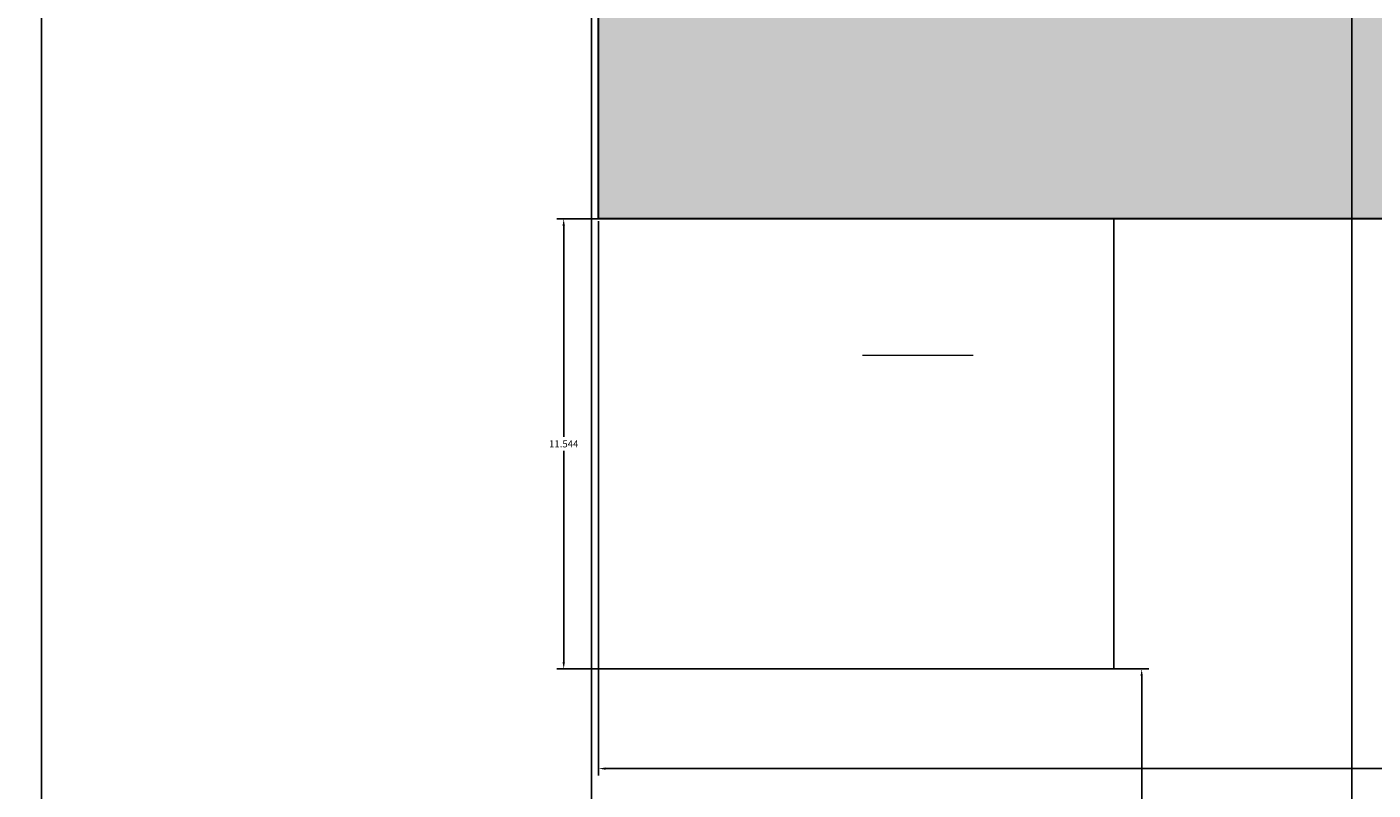
# Model space of a CAD drawing. Units: millimetres. Extents: x -8 to 285, y 5 to 221.
# Tile 11 of 30: x -8 to 27, y 131 to 150. Entities that reach past the tile are written whole.
import ezdxf

# ---------------------------------------------------------------- set-up
doc = ezdxf.new("R2010")
doc.units = ezdxf.units.MM
for name, color, linetype, lineweight in [('A-ANNO-DIMS', 2, 'Continuous', 18), ('E-ANNO-SYMB', 7, 'Continuous', 18), ('E-EQPM-PATT', 252, 'Continuous', 13), ('E-POWR-DC-NEG', 3, 'Continuous', 25), ('E-POWR-PV', 7, 'Continuous', 30)]:
    doc.layers.add(name, color=color, linetype=linetype, lineweight=lineweight)
doc.styles.get("Standard").update_dxf_attribs({"font": 'arial.ttf'})
doc.dimstyles.get("Standard").update_dxf_attribs({"dimtxt": 0.18, "dimasz": 0.18, "dimexe": 0.18, "dimexo": 0.0625, "dimgap": 0.09, "dimtad": 0, "dimtih": 1, "dimtoh": 1, "dimdec": 4, "dimzin": 0, "dimdsep": 46, "dimtxsty": 'Standard', "dimcen": 0.09, "dimadec": 0, "dimazin": 0, "dimtfac": 1, "dimtdec": 4, "dimtofl": 0, "dimtmove": 0, "dimatfit": 3, "dimfxl": 1, "dimtolj": 1, "dimtzin": 0, "dimarcsym": 0})

# ---------------------------------------------------------------- blocks, each defined once
blk = doc.blocks.new('PV-MODULE-12V')
blk.add_lwpolyline([(0, 47), (37, 47), (37, 0), (0, 0)], close=True)
blk = doc.blocks.new('*D9')
at = {"layer": 'A-ANNO-DIMS', "color": 0, "lineweight": -2, "transparency": 16777216}
for p, q in [((6.672, 133.79), (6.672, 220.737)), ((6.852, 220.557), (138.33, 220.557)), ((270.739, 220.557), (139.262, 220.557)), ((270.919, 206.519), (270.919, 220.737))]:
    blk.add_line(p, q, dxfattribs=at)
at = {"layer": 'A-ANNO-DIMS', "color": 0, "transparency": 16777216}
for points in [[(6.852, 220.587), (6.852, 220.527), (6.672, 220.557)], [(270.739, 220.587), (270.739, 220.527), (270.919, 220.557)]]:
    blk.add_solid(points, dxfattribs=at)
at = {"layer": 'Defpoints', "color": 0, "transparency": 16777216}
for p in [(270.919, 220.557), (270.919, 206.457), (6.672, 133.727)]:
    blk.add_point(p, dxfattribs=at)
at = {"layer": 'A-ANNO-DIMS', "color": 0, "transparency": 16777216, "insert": (138.796, 220.557), "char_height": 0.18, "attachment_point": 5}
blk.add_mtext('\\A1;264.25', dxfattribs=at)
blk = doc.blocks.new('*D10')
at = {"layer": 'A-ANNO-DIMS', "color": 0, "lineweight": -2, "transparency": 16777216}
for p, q in [((145.103, 206.457), (-7.608, 206.457)), ((-7.428, 206.277), (-7.428, 113.161)), ((-7.428, 19.682), (-7.428, 112.797)), ((30.453, 19.502), (-7.608, 19.502))]:
    blk.add_line(p, q, dxfattribs=at)
at = {"layer": 'A-ANNO-DIMS', "color": 0, "transparency": 16777216}
for points in [[(-7.458, 206.277), (-7.398, 206.277), (-7.428, 206.457)], [(-7.458, 19.682), (-7.398, 19.682), (-7.428, 19.502)]]:
    blk.add_solid(points, dxfattribs=at)
at = {"layer": 'Defpoints', "color": 0, "transparency": 16777216}
for p in [(-7.428, 206.457), (145.165, 206.457), (30.516, 19.502)]:
    blk.add_point(p, dxfattribs=at)
at = {"layer": 'A-ANNO-DIMS', "color": 0, "transparency": 16777216, "insert": (-7.428, 112.979), "char_height": 0.18, "attachment_point": 5}
blk.add_mtext('\\A1;186.95', dxfattribs=at)
blk = doc.blocks.new('*D11')
at = {"layer": 'A-ANNO-DIMS', "color": 0, "lineweight": -2, "transparency": 16777216}
for p, q in [((6.853, 145.209), (6.853, 130.991)), ((50.572, 145.209), (50.572, 130.991)), ((7.033, 131.171), (28.316, 131.171)), ((50.392, 131.171), (29.109, 131.171))]:
    blk.add_line(p, q, dxfattribs=at)
at = {"layer": 'A-ANNO-DIMS', "color": 0, "transparency": 16777216}
for points in [[(7.033, 131.201), (7.033, 131.141), (6.853, 131.171)], [(50.392, 131.201), (50.392, 131.141), (50.572, 131.171)]]:
    blk.add_solid(points, dxfattribs=at)
at = {"layer": 'Defpoints', "color": 0, "transparency": 16777216}
for p in [(6.853, 145.271), (50.572, 145.271), (6.853, 131.171)]:
    blk.add_point(p, dxfattribs=at)
at = {"layer": 'A-ANNO-DIMS', "color": 0, "transparency": 16777216, "insert": (28.713, 131.171), "char_height": 0.18, "attachment_point": 5}
blk.add_mtext('\\A1;43.72', dxfattribs=at)
blk = doc.blocks.new('*D18')
at = {"layer": 'A-ANNO-DIMS', "color": 0, "lineweight": -2, "transparency": 16777216}
for p, q in [((19.994, 145.271), (5.777, 145.271)), ((5.957, 145.091), (5.957, 139.681)), ((5.957, 133.907), (5.957, 139.317)), ((19.994, 133.727), (5.777, 133.727))]:
    blk.add_line(p, q, dxfattribs=at)
at = {"layer": 'A-ANNO-DIMS', "color": 0, "transparency": 16777216}
for points in [[(5.927, 145.091), (5.987, 145.091), (5.957, 145.271)], [(5.927, 133.907), (5.987, 133.907), (5.957, 133.727)]]:
    blk.add_solid(points, dxfattribs=at)
at = {"layer": 'Defpoints', "color": 0, "transparency": 16777216}
for p in [(5.957, 145.271), (20.057, 145.271), (20.057, 133.727)]:
    blk.add_point(p, dxfattribs=at)
at = {"layer": 'A-ANNO-DIMS', "color": 0, "transparency": 16777216, "insert": (5.957, 139.499), "char_height": 0.18, "attachment_point": 5}
blk.add_mtext('\\A1;11.544', dxfattribs=at)
blk = doc.blocks.new('*D19')
at = {"layer": 'A-ANNO-DIMS', "color": 0, "lineweight": -2, "transparency": 16777216}
for p, q in [((6.735, 133.727), (20.952, 133.727)), ((20.772, 133.547), (20.772, 90.056)), ((20.772, 46.201), (20.772, 89.692)), ((6.735, 46.021), (20.952, 46.021))]:
    blk.add_line(p, q, dxfattribs=at)
at = {"layer": 'A-ANNO-DIMS', "color": 0, "transparency": 16777216}
for points in [[(20.742, 133.547), (20.802, 133.547), (20.772, 133.727)], [(20.742, 46.201), (20.802, 46.201), (20.772, 46.021)]]:
    blk.add_solid(points, dxfattribs=at)
at = {"layer": 'Defpoints', "color": 0, "transparency": 16777216}
for p in [(6.672, 133.727), (6.672, 46.021), (20.772, 46.021)]:
    blk.add_point(p, dxfattribs=at)
at = {"layer": 'A-ANNO-DIMS', "color": 0, "transparency": 16777216, "insert": (20.772, 89.874), "char_height": 0.18, "attachment_point": 5}
blk.add_mtext('\\A1;87.7', dxfattribs=at)
blk = doc.blocks.new('*D24')
at = {"layer": 'A-ANNO-DIMS', "color": 0, "lineweight": -2, "transparency": 16777216}
for p, q in [((6.672, 46.084), (6.672, 220.737)), ((6.852, 220.557), (15.959, 220.557)), ((25.975, 220.557), (16.869, 220.557)), ((26.155, 65.791), (26.155, 220.737))]:
    blk.add_line(p, q, dxfattribs=at)
at = {"layer": 'A-ANNO-DIMS', "color": 0, "transparency": 16777216}
for points in [[(6.852, 220.587), (6.852, 220.527), (6.672, 220.557)], [(25.975, 220.587), (25.975, 220.527), (26.155, 220.557)]]:
    blk.add_solid(points, dxfattribs=at)
at = {"layer": 'Defpoints', "color": 0, "transparency": 16777216}
for p in [(26.155, 220.557), (26.155, 65.728), (6.672, 46.021)]:
    blk.add_point(p, dxfattribs=at)
at = {"layer": 'A-ANNO-DIMS', "color": 0, "transparency": 16777216, "insert": (16.414, 220.557), "char_height": 0.18, "attachment_point": 5}
blk.add_mtext('\\A1;19.483', dxfattribs=at)

msp = doc.modelspace()

# ---------------------------------------------------------------- hatches: boundary and pattern name
at = {"layer": 'E-EQPM-PATT'}
h = msp.add_hatch(color=256, dxfattribs=at)
h.set_gradient(color2=(0, 0, 0), tint=1)
h.paths.add_polyline_path([(6.8535, 192.2715), (6.8535, 145.2715), (43.8535, 145.2715), (43.8535, 192.2715)])
h.paths.add_polyline_path([(37.8535, 186.2715), (37.8535, 151.2715), (12.8535, 151.2715), (12.8535, 186.2715)], flags=0)
h.paths.add_polyline_path([(50.5716, 145.2715), (87.5716, 145.2715), (87.5716, 192.2715), (50.5716, 192.2715)])
h.paths.add_polyline_path([(56.5716, 186.2715), (81.5716, 186.2715), (81.5716, 151.2715), (56.5716, 151.2715)], flags=0)
h.paths.add_polyline_path([(37.8535, 176.7715), (37.8535, 186.2715), (25.3535, 186.2715), (25.3535, 176.7715)], flags=0)
h.paths.add_polyline_path([(37.8535, 176.7715), (37.8535, 186.2715), (12.8535, 186.2715), (12.8535, 176.7715)], flags=0)
h.paths.add_polyline_path([(25.3535, 160.7715), (37.8535, 160.7715), (37.8535, 186.2715), (25.3535, 186.2715)], flags=0)
h.paths.add_polyline_path([(12.8535, 151.2715), (37.8535, 151.2715), (37.8535, 186.2715), (12.8535, 186.2715)], flags=16)
h.paths.add_polyline_path([(56.5716, 186.2715), (56.5716, 160.7715), (81.5716, 160.7715), (81.5716, 186.2715)], flags=0)
h.paths.add_polyline_path([(56.5716, 151.2715), (81.5716, 151.2715), (81.5716, 186.2715), (56.5716, 186.2715)], flags=16)

# ---------------------------------------------------------------- linework, layer by layer
at = {"layer": 'E-ANNO-SYMB'}
msp.add_line((13.6122, 141.7706), (16.4517, 141.7706), dxfattribs=at)
at = {"layer": 'E-POWR-DC-NEG'}
msp.add_lwpolyline([(46.1717, 67.9064), (46.1717, 46.0211), (6.6725, 46.0211), (6.6725, 133.7273), (20.0566, 133.7273), (20.0566, 145.2715)], dxfattribs=at)

# ---------------------------------------------------------------- block references
at = {"layer": 'E-POWR-PV'}
msp.add_blockref('PV-MODULE-12V', (6.853, 145.271), dxfattribs=at)

# ---------------------------------------------------------------- dimensions: what is measured, and where the dimension line sits
at = {"layer": 'A-ANNO-DIMS'}
for base, p1, p2, override, picture, middle in [((270.9192, 220.5568), (6.6725, 133.7273), (270.9192, 206.4568), {"dimdec": 2, "dimlfac": 1, "dimrnd": 0, "dimzin": 0, "dimdsep": 46, "dimlunit": 2}, '*D9', (138.7958, 220.5568)), ((26.1554, 220.5568), (6.6725, 46.0211), (26.1554, 65.7282), {"dimdec": 3, "dimlfac": 1, "dimrnd": 0, "dimzin": 0, "dimdsep": 46, "dimlunit": 2}, '*D24', (16.4139, 220.5568))]:
    dim = msp.add_linear_dim(base=base, p1=p1, p2=p2, dimstyle='Standard', override=override, dxfattribs=at)
    dim.commit()
    dim.dimension.update_dxf_attribs({"geometry": picture, "text_midpoint": middle})
for base, p1, p2, angle, override, picture, middle in [((-7.4275, 206.4568), (30.516, 19.502), (145.1651, 206.4568), 90, {"dimdec": 2, "dimlfac": 1, "dimrnd": 0, "dimzin": 0, "dimdsep": 46, "dimlunit": 2}, '*D10', (-7.4275, 112.9794)), ((5.9566, 145.2715), (20.0566, 133.7273), (20.0566, 145.2715), 90, {"dimdec": 3, "dimlfac": 1, "dimrnd": 0, "dimzin": 0, "dimdsep": 46, "dimlunit": 2}, '*D18', (5.9566, 139.4994)), ((6.8535, 131.1715), (50.5716, 145.2715), (6.8535, 145.2715), 180, {"dimdec": 2, "dimlfac": 1, "dimrnd": 0, "dimzin": 0, "dimdsep": 46, "dimlunit": 2}, '*D11', (28.7125, 131.1715)), ((20.7725, 46.0211), (6.6725, 133.7273), (6.6725, 46.0211), 270, {"dimdec": 1, "dimlfac": 1, "dimrnd": 0, "dimzin": 0, "dimdsep": 46, "dimlunit": 2}, '*D19', (20.7725, 89.8742))]:
    dim = msp.add_linear_dim(base=base, p1=p1, p2=p2, angle=angle, dimstyle='Standard', override=override, dxfattribs=at)
    dim.commit()
    dim.dimension.update_dxf_attribs({"geometry": picture, "text_midpoint": middle})

doc.saveas('drawing.dxf')
